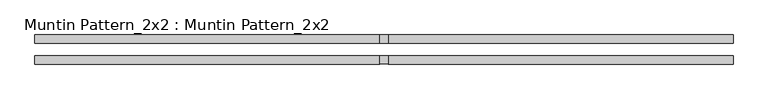
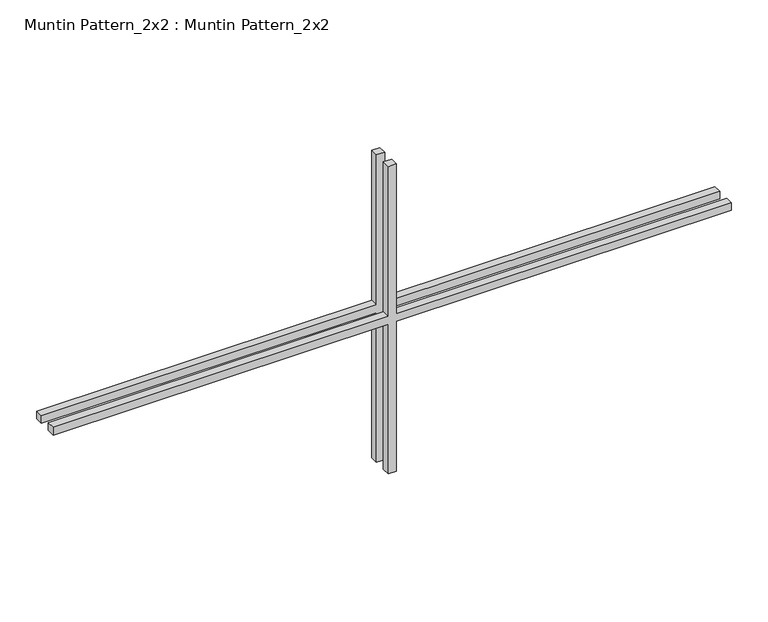
"""IFC4 building model written with IfcOpenShell, lengths in millimetres: proxy geometry, Muntin Pattern_2x2 : Muntin Pattern_2x2."""

from ifc_helpers import new_model, si_unit, frame, origin, place, context, project, spatial, polyline, outline, extrude, source, transform, mapped, element, save


def muntin_pattern_2x2_muntin_pattern_2x2_1e1a1b39(model_context):
    return source(origin(), model_context, "Body", "SweptSolid", [
        extrude(outline(polyline([(261.9375, -6.35), (261.9375, -533.4), (249.2375, -533.4), (249.2375, -6.35), (0.0, -6.35), (0.0, 6.35), (249.2375, 6.35), (249.2375, 533.4), (261.9375, 533.4), (261.9375, 6.35), (511.175, 6.35), (511.175, -6.35), (261.9375, -6.35)])), frame((0.0, 9.525, 0.0), z_axis=(0.0, 1.0, 0.0), x_axis=(0.0, 0.0, 1.0)), (0.0, 0.0, 1.0), 12.7),
        extrude(outline(polyline([(261.9375, -6.35), (261.9375, -533.4), (249.2375, -533.4), (249.2375, -6.35), (0.0, -6.35), (0.0, 6.35), (249.2375, 6.35), (249.2375, 533.4), (261.9375, 533.4), (261.9375, 6.35), (511.175, 6.35), (511.175, -6.35), (261.9375, -6.35)])), frame((0.0, -22.225, 0.0), z_axis=(0.0, 1.0, 0.0), x_axis=(0.0, 0.0, 1.0)), (0.0, 0.0, 1.0), 12.7),
    ])


if __name__ == "__main__":
    model = new_model("IFC4")
    model_context = context("Model", 3, world=origin())
    ifc_project = project(units=[si_unit("LENGTHUNIT", "METRE", prefix="MILLI")], contexts=[model_context])
    site = spatial("IfcSite", under=ifc_project)
    building = spatial("IfcBuilding", under=site)
    placement = place(None, origin())
    muntin_pattern_2x2_muntin_pattern_2x2_shape = muntin_pattern_2x2_muntin_pattern_2x2_1e1a1b39(model_context)
    element("IfcBuildingElementProxy", 1, Name="Muntin Pattern_2x2 : Muntin Pattern_2x2", ObjectType="Muntin Pattern_2x2 : Muntin Pattern_2x2", at=placement, inside=building, context=model_context, shape_type="MappedRepresentation", body=[
        mapped(muntin_pattern_2x2_muntin_pattern_2x2_shape, transform((0.0, 0.0, 0.0), x_axis=(1.0, 0.0, 0.0), y_axis=(0.0, 1.0, 0.0), z_axis=(0.0, 0.0, 1.0))),
    ])
    save(model, "model.ifc")

# Revit data of these elements
# Type "Muntin Pattern_2x2 : Muntin Pattern_2x2"
#   Width [instance default] = 4' - 0"
#   Thickness = 0' - 0 1/2"
#   Height [instance default] = 4' - 0"
#   Distance = 0' - 0 3/4"
#   Interior Material [instance default] = none
#   Exterior Material [instance default] = none
#   Default Elevation = 0
# Element 1 (IfcBuildingElementProxy, "Muntin Pattern_2x2 : Muntin Pattern_2x2")
#   Width = 3' - 6"
#   Height = 1' - 8 1/8"
#   Interior Material = Wood - Stained
#   Exterior Material = Clad - White
#   Materials on its faces: "Clad - White", "Wood - Stained"
# Materials
#   "Clad - White": class "Wood", colour RGB 242 242 238, transparency 0, Cost = 0
#   "Wood - Stained": class "Wood", colour RGB 224 178 126, transparency 0, Cost = 0
